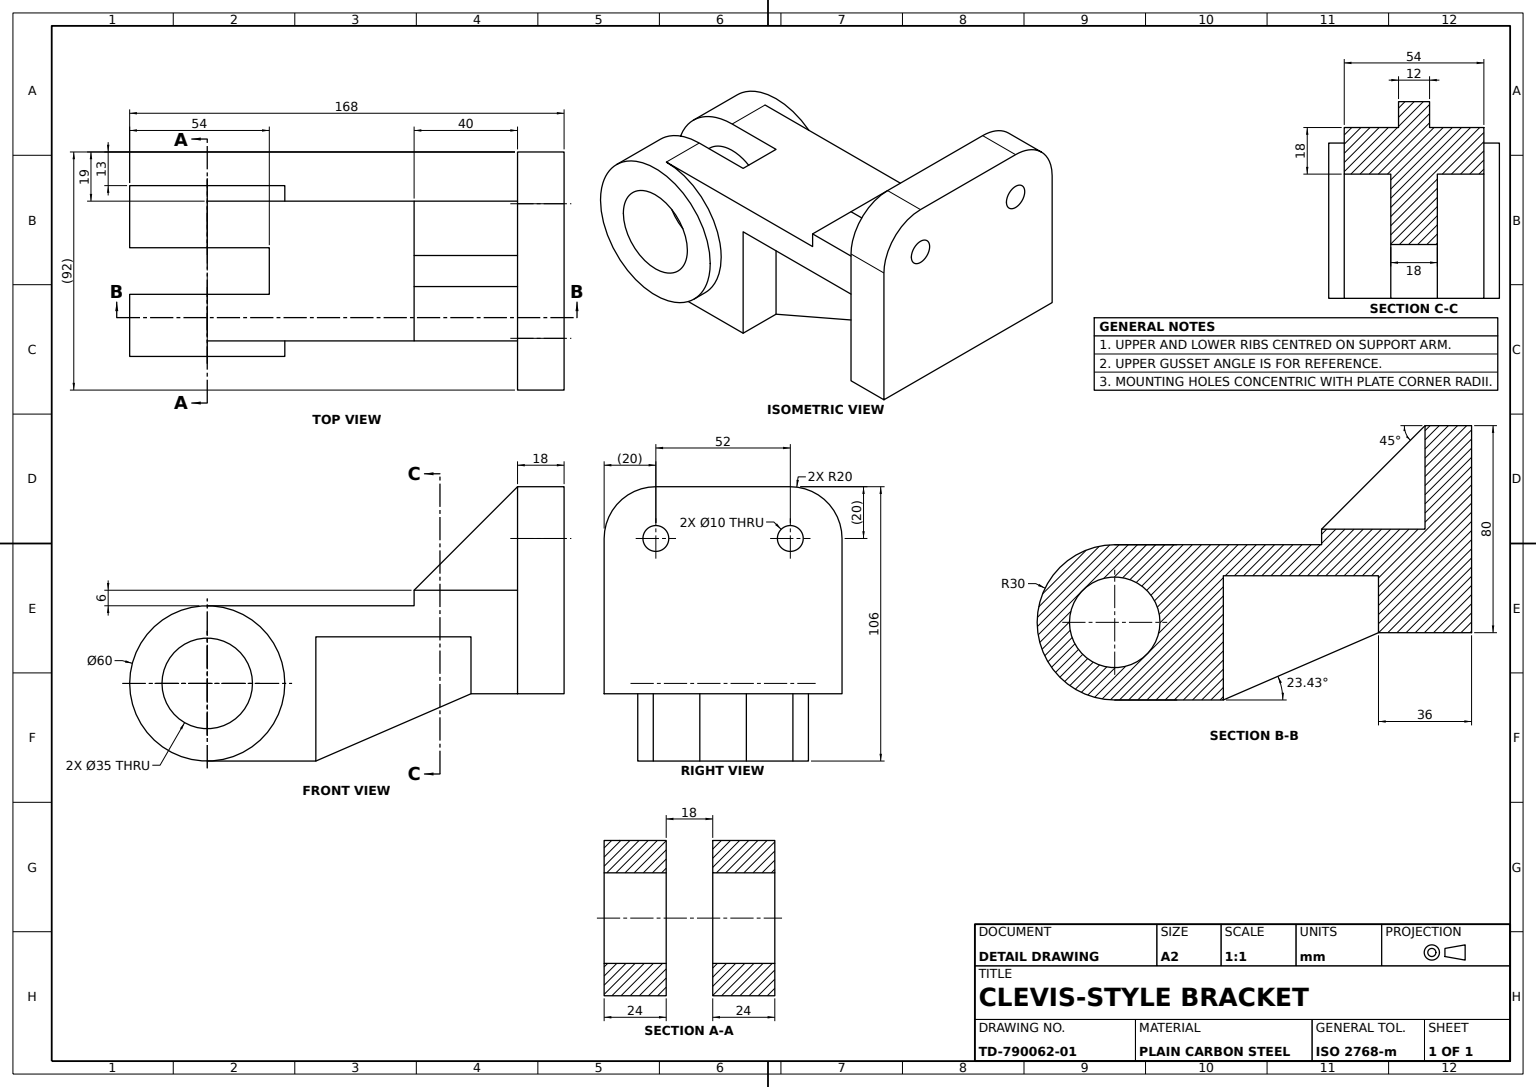
SolidWorks part; units mm, degrees
material "Plain Carbon Steel"
ref_plane "Front Plane" through (0, 0, 0) normal (0, 0, 1) x (1, 0, 0)
ref_plane "Top Plane" through (0, 0, 0) normal (0, 1, 0) x (1, 0, 0)
ref_plane "Right Plane" through (0, 0, 0) normal (1, 0, 0) x (0, 0, -1)
sketch "Hub Profile" plane through (0, 0, 0) normal (0, 0, 1) x (1, 0, 0)
  circle A0 centre (0, 0) radius 30
  circle A1 centre (0, 0) radius 17.5
  dimension "D1" = 60
  dimension "D2" = 35
extrude "Bearing Hub Ø60 Bore Ø35" add sketch "Hub Profile" along normal mid plane 66
sketch "Support Arm Profile" plane through (0, 0, 0) normal (0, 0, 1) x (1, 0, 0)
  line L1 (0, 30) -> (45.6885, 30)
  line L3 (0, -30) -> (42, -30)
  line L4 (42, 18) -> (42, -30)
  line L5 (45.6885, 30) -> (80, 30)
  line L7 (42, 18) -> (102, 18)
  line L9 (120, 36) -> (80, 36)
  line L12 (80, 36) -> (80, 30)
  line L18 (120, -4) -> (102, -4)
  line L19 (102, -4) -> (102, 18)
  line L20 (24, 30) -> (24, 56.8304) construction
  line L21 (120, 36) -> (120, -4)
  circle A0 centre (0, 0) radius 30 construction
  arc A1 (0, -30) -> (0, 30) centre (0, 0) ccw
  dimension "D1" = 12
  dimension "D2" = 18
  dimension "D3" = 6
  dimension "D4" = 40
  dimension "D5" = 120
  dimension "D6" = 60
  dimension "D7" = 74.3115
  dimension "D8" = 24
  dimension "D9" = 40
extrude "Support Arm" add sketch "Support Arm Profile" along normal mid plane 54
sketch "Hub Rib Sketch" plane through (0, 0, 0) normal (0, 0, 1) x (1, 0, 0)
  line L0 (42, -30) -> (102, -4)
rib "Hub Rib 18" sketch "Hub Rib Sketch" sketch "Hub Rib Sketch" thickness 18 extrusion direction parallel to sketch draft on no parameters "D1"=18
sketch "Mounting Plate Profile" plane through (120, 0, 0) normal (1, 0, 0) x (0, 0, -1)
  line L0 (-27, 36) -> (27, 36) construction
  line L1 (-46, -4) -> (46, -4)
  line L2 (-46, -4) -> (-46, 56)
  line L3 (-26, 76) -> (26, 76)
  line L4 (46, -4) -> (46, 56)
  arc A0 (26, 76) -> (46, 56) centre (26, 56) cw
  arc A1 (-46, 56) -> (-26, 76) centre (-26, 56) cw
  circle A2 centre (-26, 56) radius 5
  circle A3 centre (26, 56) radius 5
  point P7 (0, -4)
  point P8 (0, 76)
  point P13 (-46, 76)
  dimension "D3" = 20
  dimension "D4" = 10
  dimension "D1" = 80
  dimension "D2" = 40
  dimension "D5" = 52
extrude "Mounting Plate" add sketch "Mounting Plate Profile" along normal blind 18
sketch "Plate Rib Sketch" plane through (0, 0, 0) normal (0, 0, 1) x (1, 0, 0)
  line L0 (80, 36) -> (120, 76)
rib "Plate Rib 12" sketch "Plate Rib Sketch" sketch "Plate Rib Sketch" thickness 12 extrusion direction parallel to sketch draft on no parameters "D1"=12
sketch "Fork Slot Profile" plane through (0, 30, 0) normal (0, 1, 0) x (1, 0, 0)
  line L0 (-33.6387, 9) -> (24, 9)
  line L1 (24, 9) -> (24, -9)
  line L2 (24, -9) -> (-33.6387, -9)
  line L3 (-33.6387, -9) -> (-33.6387, 9)
  line L4 (80, -27) -> (80, 27) construction
  point P2 (24, 0)
  dimension "D1" = 24
  dimension "D2" = 18
  dimension "D3" = 113.6387
extrude "Fork Slot 24x18" cut sketch "Fork Slot Profile" against normal through all
